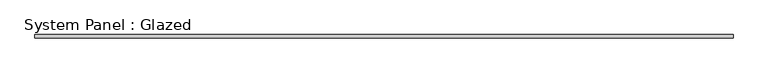
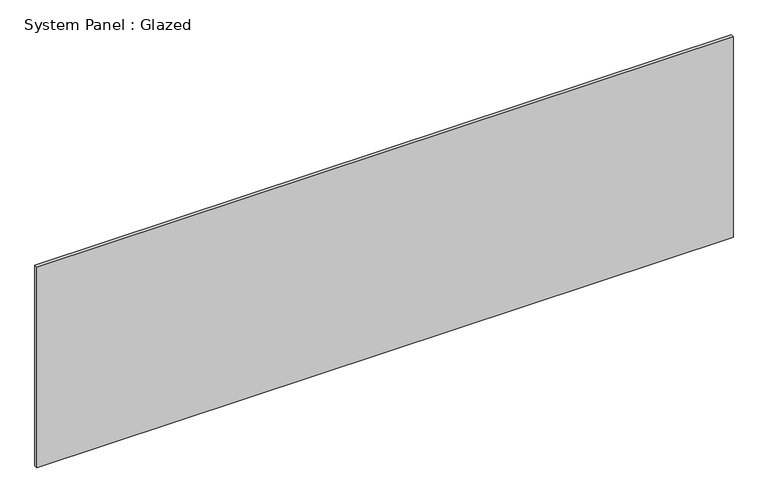
"""IFC4 building model written with IfcOpenShell, lengths in millimetres: plate geometry, System Panel : Glazed."""

from ifc_helpers import new_model, si_unit, origin, origin_with_axes, place, context, project, spatial, polyline, outline, extrude, source, transform, mapped, element, save


def system_panel_glazed_aa9a1819(model_context):
    return source(origin(), model_context, "Body", "SweptSolid", [
        extrude(outline(polyline([(2502.076725, 19.05), (-2502.076725, 19.05), (-2502.076725, 44.45), (2502.076725, 44.45), (2502.076725, 19.05)])), origin_with_axes(), (0.0, 0.0, 1.0), 1524.0),
    ])


if __name__ == "__main__":
    model = new_model("IFC4")
    model_context = context("Model", 3, world=origin())
    ifc_project = project(units=[si_unit("LENGTHUNIT", "METRE", prefix="MILLI")], contexts=[model_context])
    site = spatial("IfcSite", under=ifc_project)
    building = spatial("IfcBuilding", under=site)
    placement = place(None, origin())
    system_panel_glazed_shape = system_panel_glazed_aa9a1819(model_context)
    element("IfcPlate", 1, ObjectType="System Panel : Glazed", at=placement, inside=building, context=model_context, shape_type="MappedRepresentation", body=[
        mapped(system_panel_glazed_shape, transform((0.0, 0.0, 0.0), x_axis=(1.0, 0.0, 0.0), y_axis=(0.0, 1.0, 0.0), z_axis=(0.0, 0.0, 1.0))),
    ])
    save(model, "model.ifc")

# Revit data of these elements
# Type "System Panel : Glazed"
#   Construction Type Id = "GSP4R"
#   Analytic Construction = "1/8 in Pilkington single glazing"
#   Visual Light Transmittance = 0.9
#   Solar Heat Gain Coefficient = 0.86
#   Heat Transfer Coefficient (U) = 1.18115 BTU/(h·ft²·°F)
# Element 1 (IfcPlate, "System Panel : Glazed")
#   Materials on its faces: "Glass"
# Materials
#   "Glass": class "Glass", colour RGB 0 128 192, transparency 0.75, Description = "Soda Lime Glass", Cost = 0
